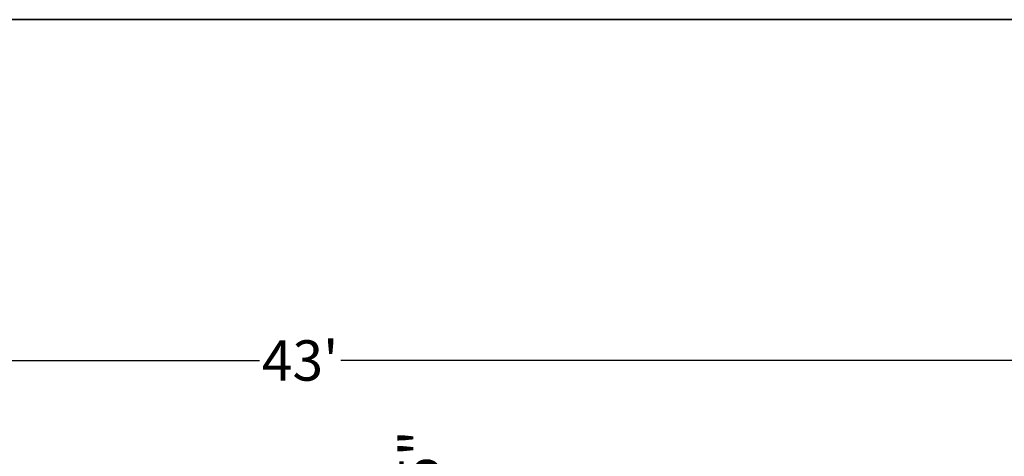
# Model space of a CAD drawing. Units: inches. Extents: x -269 to 4574, y -694 to 313.
# Tile 15 of 19: x 151 to 395, y 90 to 198. Entities that reach past the tile are written whole.
import ezdxf

# ---------------------------------------------------------------- set-up
doc = ezdxf.new("R2010")
doc.units = ezdxf.units.IN
doc.header["$MEASUREMENT"] = 0
doc.layers.add('BORDER', color=7, linetype='Continuous', lineweight=35)
doc.layers.add('DIMENSION', color=5, linetype='Continuous', lineweight=18)
doc.dimstyles.get("Standard").update_dxf_attribs({"dimtxt": 10, "dimasz": 0.18, "dimexe": 0.18, "dimexo": 0.0625, "dimgap": 0.09, "dimtad": 0, "dimdec": 1, "dimzin": 0, "dimdsep": 46, "dimlunit": 3, "dimtxsty": 'Standard', "dimcen": 0.09, "dimclrt": 7, "dimadec": 0, "dimazin": 0, "dimtfac": 1, "dimtdec": 1, "dimtofl": 0, "dimtmove": 0, "dimatfit": 3, "dimfxl": 1, "dimtolj": 1, "dimtzin": 0, "dimarcsym": 0})

# ---------------------------------------------------------------- blocks, each defined once
blk = doc.blocks.new('*D32')
at = {"layer": 'Defpoints', "color": 0, "lineweight": 0, "transparency": 16777216}
for p in [(-37.71, 113.85), (478.29, 113.67), (478.29, 113.64)]:
    blk.add_point(p, dxfattribs=at)
at = {"layer": 'DIMENSION', "color": 0, "lineweight": -2, "transparency": 16777216}
for p, q in [((-37.71, 113.79), (-37.71, 113.46)), ((-37.53, 113.64), (210.2, 113.64)), ((478.11, 113.64), (230.38, 113.64)), ((478.29, 113.61), (478.29, 113.46))]:
    blk.add_line(p, q, dxfattribs=at)
at = {"layer": 'DIMENSION', "color": 0, "lineweight": 0, "transparency": 16777216}
for points in [[(-37.53, 113.67), (-37.53, 113.61), (-37.71, 113.64)], [(478.11, 113.67), (478.11, 113.61), (478.29, 113.64)]]:
    blk.add_solid(points, dxfattribs=at)
at = {"layer": 'DIMENSION', "color": 0, "transparency": 16777216, "insert": (220.29, 113.64), "char_height": 10, "attachment_point": 5}
blk.add_mtext("\\A1;43'", dxfattribs=at)
blk = doc.blocks.new('*D65')
at = {"layer": 'Defpoints', "color": 0, "lineweight": 0, "transparency": 16777216}
for p in [(236.53, -24.12), (249.87, -24.12), (236.53, -113.07)]:
    blk.add_point(p, dxfattribs=at)
at = {"layer": 'DIMENSION', "color": 0, "lineweight": -2, "transparency": 16777216}
for p, q in [((236.59, -24.12), (250.05, -24.12)), ((249.87, -24.12), (249.87, -23.94)), ((249.87, -112.89), (249.87, -24.3)), ((236.59, -113.07), (250.05, -113.07))]:
    blk.add_line(p, q, dxfattribs=at)
at = {"layer": 'DIMENSION', "color": 0, "lineweight": 0, "transparency": 16777216}
for points in [[(249.84, -24.3), (249.9, -24.3), (249.87, -24.12)], [(249.84, -112.89), (249.9, -112.89), (249.87, -113.07)]]:
    blk.add_solid(points, dxfattribs=at)
at = {"layer": 'DIMENSION', "color": 7, "transparency": 16777216, "insert": (249.87, 42.82), "char_height": 10, "attachment_point": 5, "rotation": 90}
blk.add_mtext('\\A1;DINING SET 7\'-5"', dxfattribs=at)

msp = doc.modelspace()

# ---------------------------------------------------------------- linework, layer by layer
at = {"layer": 'BORDER'}
msp.add_lwpolyline([(-268.51, 198.09), (666.62, 198.09), (666.62, -693.82), (-268.51, -693.82)], close=True, dxfattribs=at)

# ---------------------------------------------------------------- dimensions: what is measured, and where the dimension line sits
at = {"layer": 'DIMENSION'}
dim = msp.add_linear_dim(base=(478.29, 113.64), p1=(-37.71, 113.85), p2=(478.29, 113.67), dimstyle='Standard', override={"dimclrd": 0, "dimclre": 0, "dimclrt": 0}, dxfattribs=at)
dim.commit()
dim.dimension.update_dxf_attribs({"geometry": '*D32', "text_midpoint": (220.29, 113.64)})
dim = msp.add_linear_dim(base=(249.8693, -24.1158), p1=(236.5257, -113.0737), p2=(236.5257, -24.1158), angle=90, text='DINING SET <>', dimstyle='Standard', override={"dimdec": 1, "dimlfac": 1, "dimrnd": 0, "dimzin": 1, "dimdsep": 46, "dimlunit": 4, "dimfrac": 2}, dxfattribs=at)
dim.commit()
dim.dimension.update_dxf_attribs({"geometry": '*D65', "text_midpoint": (249.8693, 42.8209)})

doc.saveas('drawing.dxf')
